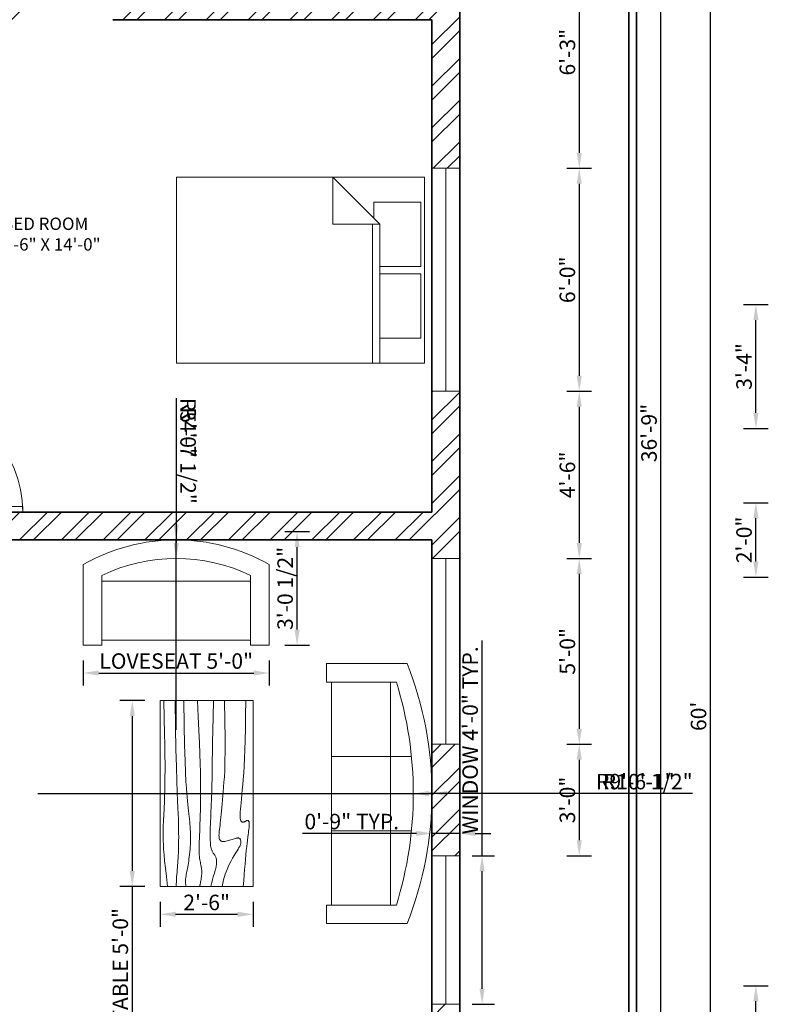
# Model space of a CAD drawing. Units: inches. Extents: x 468 to 1096, y 138 to 946.
# Tile 5 of 6: x 854 to 1096, y 448 to 766. Entities that reach past the tile are written whole.
import ezdxf

# ---------------------------------------------------------------- set-up
doc = ezdxf.new("R2010")
doc.units = ezdxf.units.IN
for name, color, linetype, lineweight in [('A-ANNO-DIMS', 2, 'Continuous', 18), ('A-AREA-IDEN', 7, 'Continuous', 18), ('A-DOOR', 3, 'Continuous', 18), ('A-FURN', 8, 'Continuous', 18), ('A-GLAZ', 4, 'Continuous', 18), ('A-WALL', 7, 'Continuous', 35), ('A-WALL-PATT', 8, 'Continuous', 13), ('C-PROP', 7, 'Continuous', 35)]:
    doc.layers.add(name, color=color, linetype=linetype, lineweight=lineweight)
doc.styles.get("Standard").update_dxf_attribs({"font": 'arial.ttf'})
doc.dimstyles.new('ISO-25', dxfattribs={"dimtxt": 5, "dimasz": 5, "dimexe": 4, "dimexo": 4, "dimtad": 1, "dimdec": 1, "dimlunit": 3, "dimtxsty": 'Standard', "dimcen": 2.5, "dimadec": 0, "dimazin": 0, "dimtfac": 1, "dimtdec": 1, "dimtmove": 0, "dimatfit": 3, "dimfxl": 4, "dimfxlon": 1, "dimarcsym": 0})

# ---------------------------------------------------------------- blocks, each defined once
blk = doc.blocks.new('*U3')
for p, q in [((0, 0), (0, -6)), ((-36, 0), (-36, -6))]:
    blk.add_line(p, q)
blk.add_lwpolyline([(0, 0), (0, 36), (-1.75, 36), (-1.75, 0)], close=True)
blk.add_arc((0, 0), 36, 90, 180)
blk = doc.blocks.new('Sofa - Roundback 7 ft.')
for p, q in [((-12.00002, -32.4421), (-12.00003, -6.5971)), ((11.99997, -32.4421), (11.99998, -6.5971)), ((-36.000027, -34), (-36.000027, -11.4696)), ((35.99998, -34), (35.99998, -11.4696)), ((-35.999844, -13.3819), (35.9998, -13.3819)), ((-36.000027, -32.4421), (35.99998, -32.4421))]:
    blk.add_line(p, q)
for points in [[(-36.000027, -34), (-42.000027, -34), (-42.000027, -8)], [(41.99998, -8), (41.99998, -34), (35.99998, -34)]]:
    blk.add_lwpolyline(points)
for centre, radius, start, end in [((0, -114.25), 114.25, 68.43141, 111.5686), ((-0.00001, -127.1968), 121.1968, 72.72033, 107.2797)]:
    blk.add_arc(centre, radius, start, end)
blk = doc.blocks.new('Sofa - Roundback Loveseat 5 ft.')
for p, q in [((0, -32.44198), (0, -5.99998)), ((-24, -33.99998), (-24, -11.46958)), ((24.00004, -33.99998), (24.00004, -11.46958)), ((-23.9998, -13.38178), (23.99986, -13.38178)), ((-24, -32.44198), (24.00004, -32.44198))]:
    blk.add_line(p, q)
for points in [[(-24, -33.99998), (-30, -33.99998), (-30, -7.99998)], [(30.00004, -7.99998), (30.00004, -33.99998), (24.00004, -33.99998)]]:
    blk.add_lwpolyline(points)
for centre, radius, start, end in [((0, -60.24998), 60.24998, 60.13715, 119.8628), ((0, -61.38438), 55.38444, 64.32083, 115.6792)]:
    blk.add_arc(centre, radius, start, end)
blk = doc.blocks.new('Table - Rectangular Woodgrain 60 x 30 in.')
for p, q in [((0, 0), (0, -30)), ((60, 0), (0, 0)), ((60, -30), (60, 0)), ((0, -30), (60, -30))]:
    blk.add_line(p, q)
for points in [[(0, -2.4), (4.8155, -2.418), (9.0302, -2.4688), (12.709, -2.5477), (15.9167, -2.65), (18.7181, -2.7711), (21.1781, -2.9063), (23.3616, -3.0508), (25.3333, -3.2), (27.1477, -3.3495), (28.8172, -3.4958), (30.3437, -3.636), (31.7291, -3.7667), (32.9756, -3.8849), (34.0849, -3.9875), (35.059, -4.0714), (35.9, -4.1334), (36.6114, -4.1711), (37.2041, -4.1854), (37.6906, -4.1779), (38.0833, -4.15), (38.3948, -4.1034), (38.6375, -4.0396), (38.8239, -3.9602), (38.9666, -3.8667), (39.0764, -3.7608), (39.1573, -3.6448), (39.2116, -3.521), (39.2416, -3.3917), (39.2498, -3.2593), (39.2385, -3.1261), (39.21, -2.9944), (39.1666, -2.8667), (39.111, -2.7447), (39.0468, -2.6281), (38.978, -2.5163), (38.9083, -2.4083), (38.8418, -2.3035), (38.7823, -2.201), (38.7337, -2.1001), (38.7, -2), (38.6844, -1.9003), (38.6875, -1.8021), (38.7094, -1.707), (38.75, -1.6167), (38.8094, -1.5326), (38.8875, -1.4563), (38.9844, -1.3893), (39.1, -1.3333), (39.2351, -1.2896), (39.3937, -1.2583), (39.5804, -1.2396), (39.8, -1.2333), (40.057, -1.2396), (40.3562, -1.2583), (40.7023, -1.2896), (41.1, -1.3333), (41.5547, -1.3895), (42.0755, -1.4573), (42.6721, -1.5361), (43.3542, -1.625), (44.1316, -1.7233), (45.014, -1.8302), (46.0114, -1.9449), (47.1333, -2.0667), (48.3862, -2.1947), (49.7625, -2.3281), (51.2513, -2.4663), (52.8416, -2.6083), (54.5226, -2.7535), (56.2833, -2.9011), (58.1127, -3.0501), (60, -3.2)], [(0, -9.2), (6.5759, -9.0858), (11.9385, -9.0365), (16.2527, -9.0418), (19.6833, -9.0917), (22.3952, -9.1759), (24.5531, -9.2844), (26.322, -9.4069), (27.8666, -9.5333), (29.3241, -9.6553), (30.7203, -9.7719), (32.0532, -9.8837), (33.3208, -9.9917), (34.5213, -10.0965), (35.6526, -10.199), (36.7128, -10.2999), (37.7, -10.4), (38.6129, -10.4996), (39.4531, -10.5969), (40.223, -10.6895), (40.925, -10.775), (41.5613, -10.8512), (42.1344, -10.9156), (42.6465, -10.966), (43.1, -11), (43.4976, -11.0158), (43.8437, -11.0136), (44.143, -10.9942), (44.4, -10.9583), (44.6195, -10.9069), (44.8062, -10.8406), (44.9648, -10.7603), (45.1, -10.6667), (45.2155, -10.5598), (45.3114, -10.4365), (45.3871, -10.2929), (45.4416, -10.125), (45.4743, -9.929), (45.4844, -9.7011), (45.4709, -9.4371), (45.4333, -9.1333), (45.3716, -8.7883), (45.2896, -8.4104), (45.1919, -8.0107), (45.0833, -7.6), (44.9685, -7.1893), (44.8521, -6.7896), (44.7388, -6.4117), (44.6333, -6.0667), (44.54, -5.7628), (44.4614, -5.4979), (44.4001, -5.2675), (44.3583, -5.0667), (44.3384, -4.8909), (44.3427, -4.7354), (44.3736, -4.5956), (44.4333, -4.4667), (44.5236, -4.3453), (44.6427, -4.2333), (44.7884, -4.1339), (44.9583, -4.05), (45.1501, -3.9849), (45.3614, -3.9417), (45.59, -3.9234), (45.8333, -3.9333), (46.0915, -3.9749), (46.3734, -4.0531), (46.6906, -4.1736), (47.0542, -4.3417), (47.4756, -4.5629), (47.9661, -4.8427), (48.5372, -5.1866), (49.2, -5.6), (49.9676, -6.0844), (50.8594, -6.625), (51.8965, -7.2031), (53.1, -7.8), (54.491, -8.3969), (56.0906, -8.975), (57.9199, -9.5156), (60, -10)], [(0, -12.8), (5.1847, -12.9322), (9.6213, -13.0323), (13.3963, -13.1059), (16.5958, -13.1583), (19.3063, -13.1952), (21.614, -13.2219), (23.6054, -13.2439), (25.3666, -13.2667), (26.9728, -13.2947), (28.4531, -13.3281), (29.8256, -13.3663), (31.1083, -13.4083), (32.3191, -13.4535), (33.476, -13.501), (34.597, -13.5501), (35.7, -13.6), (36.7984, -13.6497), (37.8875, -13.6979), (38.9578, -13.743), (40, -13.7833), (41.0047, -13.8174), (41.9625, -13.8438), (42.864, -13.8607), (43.7, -13.8667), (44.4631, -13.8604), (45.1552, -13.8417), (45.7801, -13.8104), (46.3416, -13.7667), (46.8439, -13.7104), (47.2906, -13.6417), (47.6858, -13.5604), (48.0333, -13.4667), (48.3375, -13.3608), (48.6042, -13.2448), (48.8396, -13.121), (49.05, -12.9917), (49.2417, -12.8593), (49.4208, -12.7261), (49.5937, -12.5944), (49.7667, -12.4667), (49.9452, -12.3451), (50.1323, -12.2313), (50.3303, -12.1268), (50.5416, -12.0333), (50.7686, -11.9524), (51.0135, -11.8854), (51.2788, -11.8341), (51.5666, -11.8), (51.8785, -11.7843), (52.2116, -11.7865), (52.562, -11.8059), (52.926, -11.8417), (53.2998, -11.8931), (53.6795, -11.9594), (54.0614, -12.0397), (54.4416, -12.1333), (54.8223, -12.2401), (55.2293, -12.3625), (55.6942, -12.5037), (56.2489, -12.6667), (56.9251, -12.8547), (57.7545, -13.0708), (58.7689, -13.3182), (60, -13.6)], [(0, -18), (5.124, -17.7273), (9.6609, -17.5057), (13.6705, -17.3303), (17.2125, -17.1958), (20.3467, -17.0973), (23.1328, -17.0297), (25.6307, -16.9878), (27.9, -16.9667), (29.9928, -16.9617), (31.9302, -16.9703), (33.7254, -16.9907), (35.3917, -17.0208), (36.9423, -17.0588), (38.3906, -17.1026), (39.7499, -17.1503), (41.0333, -17.2), (42.2519, -17.2496), (43.4073, -17.2969), (44.4986, -17.3395), (45.525, -17.375), (46.4858, -17.4012), (47.3802, -17.4156), (48.2074, -17.416), (48.9667, -17.4), (49.6583, -17.3662), (50.2872, -17.3167), (50.8595, -17.2547), (51.3812, -17.1833), (51.8584, -17.1057), (52.2971, -17.025), (52.7034, -16.9443), (53.0833, -16.8667), (53.443, -16.7951), (53.789, -16.7313), (54.128, -16.6768), (54.4666, -16.6334), (54.8115, -16.6024), (55.1693, -16.5854), (55.5465, -16.5841), (55.95, -16.6), (56.3828, -16.6337), (56.8346, -16.6823), (57.2915, -16.7418), (57.7396, -16.8084), (58.165, -16.878), (58.5539, -16.9469), (58.8924, -17.0111), (59.1666, -17.0667), (59.3679, -17.1107), (59.5078, -17.1438), (59.6032, -17.1675), (59.6708, -17.1833), (59.7275, -17.193), (59.7901, -17.1979), (59.8753, -17.1998), (60, -17.2)], [(0, -22.4), (8.0098, -22.2501), (14.4094, -22.1011), (19.4168, -21.9535), (23.25, -21.8083), (26.1269, -21.6663), (28.2656, -21.5281), (29.884, -21.3947), (31.2, -21.2667), (32.3967, -21.1448), (33.5172, -21.0292), (34.5697, -20.9198), (35.5625, -20.8167), (36.5037, -20.7198), (37.4015, -20.6292), (38.2642, -20.5448), (39.1, -20.4667), (39.9164, -20.3951), (40.7187, -20.3313), (41.5117, -20.2768), (42.3, -20.2333), (43.0883, -20.2024), (43.8812, -20.1854), (44.6836, -20.1841), (45.5, -20.2), (46.3328, -20.234), (47.1747, -20.2844), (48.0163, -20.3488), (48.8479, -20.425), (49.66, -20.5106), (50.4429, -20.6031), (51.1872, -20.7004), (51.8833, -20.8), (52.5246, -20.8999), (53.1166, -20.9995), (53.6681, -21.0983), (54.1875, -21.1958), (54.6834, -21.2919), (55.1646, -21.3859), (55.6394, -21.4777), (56.1167, -21.5667), (56.6028, -21.6515), (57.0961, -21.7266), (57.5929, -21.7852), (58.0896, -21.8208), (58.5823, -21.8268), (59.0674, -21.7964), (59.5412, -21.723), (60, -21.6)], [(0, -25.2), (8.6355, -25.0504), (15.7026, -24.9031), (21.4049, -24.7606), (25.9458, -24.625), (29.529, -24.4988), (32.3578, -24.3844), (34.6359, -24.284), (36.5667, -24.2), (38.3213, -24.1341), (39.9417, -24.0854), (41.437, -24.0523), (42.8167, -24.0333), (44.0901, -24.0268), (45.2667, -24.0313), (46.3557, -24.0451), (47.3667, -24.0667), (48.309, -24.0947), (49.1928, -24.1287), (50.0284, -24.168), (50.826, -24.2125), (51.5959, -24.2617), (52.3483, -24.3151), (53.0935, -24.3725), (53.8417, -24.4334), (54.6009, -24.497), (55.3699, -24.561), (56.1454, -24.6226), (56.9239, -24.6792), (57.7021, -24.7279), (58.4764, -24.7662), (59.2435, -24.7911), (60, -24.8)], [(0, -28.8), (5.6867, -28.6681), (10.45, -28.5698), (14.407, -28.5012), (17.675, -28.4584), (20.3711, -28.4374), (22.6125, -28.4344), (24.5164, -28.4455), (26.2, -28.4667), (27.762, -28.4947), (29.2276, -28.5281), (30.6033, -28.5663), (31.8958, -28.6084), (33.1118, -28.6535), (34.2578, -28.7011), (35.3405, -28.7501), (36.3666, -28.8), (37.3443, -28.8497), (38.288, -28.8974), (39.2137, -28.9412), (40.1375, -28.9792), (41.0753, -29.0093), (42.0432, -29.0297), (43.0572, -29.0384), (44.1333, -29.0333), (45.2936, -29.0114), (46.5843, -28.9641), (48.0579, -28.8816), (49.7666, -28.7542), (51.7629, -28.5721), (54.0989, -28.3255), (56.8272, -28.0048), (60, -27.6)]]:
    blk.add_lwpolyline(points)
blk = doc.blocks.new('Bed - Queen')
for p, q in [((0, -80.00003), (0, 0)), ((0, 0), (59.99999, 0)), ((59.99999, 0), (59.99999, -80.00003)), ((7.99999, -1.2), (28.79998, -1.2)), ((7.99999, -14.4), (7.99999, -1.2)), ((28.79998, -1.2), (28.79998, -14.4)), ((31.19999, -1.2), (51.99999, -1.2)), ((31.19999, -14.4), (31.19999, -1.2)), ((51.99999, -1.2), (51.99999, -16.4)), ((0, -14.4), (44.8, -14.4)), ((59.99999, -29.6), (44.8, -14.4)), ((44.8, -14.4), (44.8, -29.6)), ((44.8, -16.8), (0, -16.8)), ((51.99999, -16.4), (46.79936, -16.4)), ((44.8, -29.6), (59.99999, -29.6)), ((59.99999, -80.00003), (0, -80.00003))]:
    blk.add_line(p, q)
blk = doc.blocks.new('*D26')
at = {"layer": 'A-ANNO-DIMS', "color": 0, "lineweight": -2, "transparency": 16777216}
for p, q in [((1073, 901.16), (1081, 901.16)), ((1077, 186.16), (1077, 896.16)), ((1073, 181.16), (1081, 181.16))]:
    blk.add_line(p, q, dxfattribs=at)
at = {"layer": 'A-ANNO-DIMS', "color": 0, "transparency": 16777216}
for points in [[(1076.17, 896.16), (1077.83, 896.16), (1077, 901.16)], [(1076.17, 186.16), (1077.83, 186.16), (1077, 181.16)]]:
    blk.add_solid(points, dxfattribs=at)
at = {"layer": 'Defpoints', "color": 0, "transparency": 16777216}
for p in [(1053.13, 901.16), (1077, 901.16), (1053.13, 181.16)]:
    blk.add_point(p, dxfattribs=at)
at = {"layer": 'A-ANNO-DIMS', "color": 0, "transparency": 16777216, "insert": (1073.82, 541.16), "char_height": 5, "attachment_point": 5, "rotation": 90}
blk.add_mtext("60'", dxfattribs=at)
blk = doc.blocks.new('*D28')
at = {"layer": 'A-ANNO-DIMS', "color": 0, "lineweight": -2, "transparency": 16777216}
for p, q in [((1057.13, 853.16), (1065.02, 853.16)), ((1061.02, 417.16), (1061.02, 848.16)), ((1057.13, 412.16), (1065.02, 412.16))]:
    blk.add_line(p, q, dxfattribs=at)
at = {"layer": 'A-ANNO-DIMS', "color": 0, "transparency": 16777216}
for points in [[(1060.18, 848.16), (1061.85, 848.16), (1061.02, 853.16)], [(1060.18, 417.16), (1061.85, 417.16), (1061.02, 412.16)]]:
    blk.add_solid(points, dxfattribs=at)
at = {"layer": 'Defpoints', "color": 0, "transparency": 16777216}
for p in [(1053.13, 853.16), (1061.02, 853.16), (1053.13, 412.16)]:
    blk.add_point(p, dxfattribs=at)
at = {"layer": 'A-ANNO-DIMS', "color": 0, "transparency": 16777216, "insert": (1057.84, 632.66), "char_height": 5, "attachment_point": 5, "rotation": 90}
blk.add_mtext('36\'-9"', dxfattribs=at)
blk = doc.blocks.new('WIN-48-W9')
for p, q in [((0, 0), (0, 9)), ((48, 0), (48, 9)), ((0, 4.5), (48, 4.5))]:
    blk.add_line(p, q)
blk = doc.blocks.new('*D43')
at = {"layer": 'A-ANNO-DIMS', "color": 0, "lineweight": -2, "transparency": 16777216}
for p, q in [((1003.33, 496.16), (1003.33, 565.68)), ((1000.13, 496.16), (1007.33, 496.16)), ((1003.33, 453.16), (1003.33, 491.16)), ((1000.13, 448.16), (1007.33, 448.16))]:
    blk.add_line(p, q, dxfattribs=at)
at = {"layer": 'A-ANNO-DIMS', "color": 0, "transparency": 16777216}
for points in [[(1002.5, 491.16), (1004.16, 491.16), (1003.33, 496.16)], [(1002.5, 453.16), (1004.16, 453.16), (1003.33, 448.16)]]:
    blk.add_solid(points, dxfattribs=at)
at = {"layer": 'Defpoints', "color": 0, "transparency": 16777216}
for p in [(996.13, 496.16), (1003.33, 496.16), (996.13, 448.16)]:
    blk.add_point(p, dxfattribs=at)
at = {"layer": 'A-ANNO-DIMS', "color": 0, "transparency": 16777216, "insert": (1000.12, 533.42), "char_height": 5, "attachment_point": 5, "rotation": 90}
blk.add_mtext('WINDOW 4\'-0" TYP.', dxfattribs=at)
blk = doc.blocks.new('*D44')
at = {"layer": 'A-ANNO-DIMS', "color": 0, "lineweight": -2, "transparency": 16777216}
for p, q in [((987.13, 500.16), (987.13, 507.36)), ((996.13, 500.16), (996.13, 507.36)), ((982.13, 503.36), (945.4, 503.36)), ((996.13, 503.36), (987.13, 503.36)), ((1001.13, 503.36), (1006.13, 503.36))]:
    blk.add_line(p, q, dxfattribs=at)
at = {"layer": 'A-ANNO-DIMS', "color": 0, "transparency": 16777216}
for points in [[(982.13, 504.19), (982.13, 502.53), (987.13, 503.36)], [(1001.13, 504.19), (1001.13, 502.53), (996.13, 503.36)]]:
    blk.add_solid(points, dxfattribs=at)
at = {"layer": 'Defpoints', "color": 0, "transparency": 16777216}
for p in [(987.13, 503.36), (987.13, 496.16), (996.13, 496.16)]:
    blk.add_point(p, dxfattribs=at)
at = {"layer": 'A-ANNO-DIMS', "color": 0, "transparency": 16777216, "insert": (961.27, 506.54), "char_height": 5, "attachment_point": 5}
blk.add_mtext('0\'-9" TYP.', dxfattribs=at)
blk = doc.blocks.new('*D49')
at = {"layer": 'A-ANNO-DIMS', "color": 0, "lineweight": -2, "transparency": 16777216}
for p, q in [((874.63, 559.16), (874.63, 551.16)), ((934.63, 559.16), (934.63, 551.16)), ((879.63, 555.16), (929.63, 555.16))]:
    blk.add_line(p, q, dxfattribs=at)
at = {"layer": 'A-ANNO-DIMS', "color": 0, "transparency": 16777216}
for points in [[(879.63, 555.99), (879.63, 554.33), (874.63, 555.16)], [(929.63, 555.99), (929.63, 554.33), (934.63, 555.16)]]:
    blk.add_solid(points, dxfattribs=at)
at = {"layer": 'Defpoints', "color": 0, "transparency": 16777216}
for p in [(874.63, 564.16), (934.63, 564.16), (934.63, 555.16)]:
    blk.add_point(p, dxfattribs=at)
at = {"layer": 'A-ANNO-DIMS', "color": 0, "transparency": 16777216, "insert": (904.63, 558.37), "char_height": 5, "attachment_point": 5}
blk.add_mtext('LOVESEAT 5\'-0"', dxfattribs=at)
blk = doc.blocks.new('*D50')
at = {"layer": 'A-ANNO-DIMS', "color": 0, "lineweight": -2, "transparency": 16777216}
for p, q in [((939.63, 600.83), (947.63, 600.83)), ((943.63, 569.16), (943.63, 595.83)), ((939.63, 564.16), (947.63, 564.16))]:
    blk.add_line(p, q, dxfattribs=at)
at = {"layer": 'A-ANNO-DIMS', "color": 0, "transparency": 16777216}
for points in [[(942.8, 595.83), (944.46, 595.83), (943.63, 600.83)], [(942.8, 569.16), (944.46, 569.16), (943.63, 564.16)]]:
    blk.add_solid(points, dxfattribs=at)
at = {"layer": 'Defpoints', "color": 0, "transparency": 16777216}
for p in [(934.63, 600.83), (943.63, 600.83), (934.63, 564.16)]:
    blk.add_point(p, dxfattribs=at)
at = {"layer": 'A-ANNO-DIMS', "color": 0, "transparency": 16777216, "insert": (940.42, 582.49), "char_height": 5, "attachment_point": 5, "rotation": 90}
blk.add_mtext('3\'-0 1/2"', dxfattribs=at)
blk = doc.blocks.new('*D51')
at = {"layer": 'A-ANNO-DIMS', "color": 0, "lineweight": -2, "transparency": 16777216}
for p, q in [((894.45, 546.23), (886.45, 546.23)), ((890.45, 541.23), (890.45, 491.23)), ((894.45, 486.23), (886.45, 486.23)), ((890.45, 486.23), (890.45, 411.4))]:
    blk.add_line(p, q, dxfattribs=at)
at = {"layer": 'A-ANNO-DIMS', "color": 0, "transparency": 16777216}
for points in [[(889.62, 541.23), (891.28, 541.23), (890.45, 546.23)], [(889.62, 491.23), (891.28, 491.23), (890.45, 486.23)]]:
    blk.add_solid(points, dxfattribs=at)
at = {"layer": 'Defpoints', "color": 0, "transparency": 16777216}
for p in [(899.45, 546.23), (890.45, 486.23), (899.45, 486.23)]:
    blk.add_point(p, dxfattribs=at)
at = {"layer": 'A-ANNO-DIMS', "color": 0, "transparency": 16777216, "insert": (887.24, 446.31), "char_height": 5, "attachment_point": 5, "rotation": 90}
blk.add_mtext('LOUNGE TABLE 5\'-0"', dxfattribs=at)
blk = doc.blocks.new('*D52')
at = {"layer": 'A-ANNO-DIMS', "color": 0, "lineweight": -2, "transparency": 16777216}
for p, q in [((899.45, 481.23), (899.45, 473.23)), ((929.45, 481.23), (929.45, 473.23)), ((904.45, 477.23), (924.45, 477.23))]:
    blk.add_line(p, q, dxfattribs=at)
at = {"layer": 'A-ANNO-DIMS', "color": 0, "transparency": 16777216}
for points in [[(904.45, 478.06), (904.45, 476.39), (899.45, 477.23)], [(924.45, 478.06), (924.45, 476.39), (929.45, 477.23)]]:
    blk.add_solid(points, dxfattribs=at)
at = {"layer": 'Defpoints', "color": 0, "transparency": 16777216}
for p in [(899.45, 486.23), (929.45, 486.23), (929.45, 477.23)]:
    blk.add_point(p, dxfattribs=at)
at = {"layer": 'A-ANNO-DIMS', "color": 0, "transparency": 16777216, "insert": (914.45, 480.41), "char_height": 5, "attachment_point": 5}
blk.add_mtext('2\'-6"', dxfattribs=at)
blk = doc.blocks.new('*D64')
at = {"layer": 'A-ANNO-DIMS', "color": 0, "lineweight": -2, "transparency": 16777216}
for p, q in [((854.13, 146.61), (854.13, 138.61)), ((884.13, 146.61), (884.13, 138.61)), ((859.13, 142.61), (879.13, 142.61))]:
    blk.add_line(p, q, dxfattribs=at)
at = {"layer": 'A-ANNO-DIMS', "color": 0, "transparency": 16777216}
for points in [[(859.13, 143.44), (859.13, 141.78), (854.13, 142.61)], [(879.13, 143.44), (879.13, 141.78), (884.13, 142.61)]]:
    blk.add_solid(points, dxfattribs=at)
at = {"layer": 'Defpoints', "color": 0, "transparency": 16777216}
for p in [(854.13, 766.16), (884.13, 766.16), (884.13, 142.61)]:
    blk.add_point(p, dxfattribs=at)
at = {"layer": 'A-ANNO-DIMS', "color": 0, "transparency": 16777216, "insert": (869.13, 145.79), "char_height": 5, "attachment_point": 5}
blk.add_mtext('2\'-6"', dxfattribs=at)
blk = doc.blocks.new('*D67')
at = {"layer": 'A-ANNO-DIMS', "color": 0, "lineweight": -2, "transparency": 16777216}
for p, q in [((1030.68, 718.16), (1038.68, 718.16)), ((1034.68, 713.16), (1034.68, 651.16)), ((1030.68, 646.16), (1038.68, 646.16))]:
    blk.add_line(p, q, dxfattribs=at)
at = {"layer": 'A-ANNO-DIMS', "color": 0, "transparency": 16777216}
for points in [[(1033.85, 713.16), (1035.51, 713.16), (1034.68, 718.16)], [(1033.85, 651.16), (1035.51, 651.16), (1034.68, 646.16)]]:
    blk.add_solid(points, dxfattribs=at)
at = {"layer": 'Defpoints', "color": 0, "transparency": 16777216}
for p in [(996.13, 718.16), (996.13, 646.16), (1034.68, 646.16)]:
    blk.add_point(p, dxfattribs=at)
at = {"layer": 'A-ANNO-DIMS', "color": 0, "transparency": 16777216, "insert": (1031.5, 682.16), "char_height": 5, "attachment_point": 5, "rotation": 90}
blk.add_mtext('6\'-0"', dxfattribs=at)
blk = doc.blocks.new('*D68')
at = {"layer": 'A-ANNO-DIMS', "color": 0, "lineweight": -2, "transparency": 16777216}
for p, q in [((1030.68, 592.16), (1038.68, 592.16)), ((1034.68, 587.16), (1034.68, 537.16)), ((1030.68, 532.16), (1038.68, 532.16))]:
    blk.add_line(p, q, dxfattribs=at)
at = {"layer": 'A-ANNO-DIMS', "color": 0, "transparency": 16777216}
for points in [[(1033.85, 587.16), (1035.51, 587.16), (1034.68, 592.16)], [(1033.85, 537.16), (1035.51, 537.16), (1034.68, 532.16)]]:
    blk.add_solid(points, dxfattribs=at)
at = {"layer": 'Defpoints', "color": 0, "transparency": 16777216}
for p in [(996.13, 592.16), (996.13, 532.16), (1034.68, 532.16)]:
    blk.add_point(p, dxfattribs=at)
at = {"layer": 'A-ANNO-DIMS', "color": 0, "transparency": 16777216, "insert": (1031.5, 562.16), "char_height": 5, "attachment_point": 5, "rotation": 90}
blk.add_mtext('5\'-0"', dxfattribs=at)
blk = doc.blocks.new('*D69')
at = {"layer": 'A-ANNO-DIMS', "color": 0, "lineweight": -2, "transparency": 16777216}
for p, q in [((1030.68, 532.16), (1038.68, 532.16)), ((1034.68, 527.16), (1034.68, 501.16)), ((1030.68, 496.16), (1038.68, 496.16))]:
    blk.add_line(p, q, dxfattribs=at)
at = {"layer": 'A-ANNO-DIMS', "color": 0, "transparency": 16777216}
for points in [[(1033.85, 527.16), (1035.51, 527.16), (1034.68, 532.16)], [(1033.85, 501.16), (1035.51, 501.16), (1034.68, 496.16)]]:
    blk.add_solid(points, dxfattribs=at)
at = {"layer": 'Defpoints', "color": 0, "transparency": 16777216}
for p in [(996.13, 532.16), (996.13, 496.16), (1034.68, 496.16)]:
    blk.add_point(p, dxfattribs=at)
at = {"layer": 'A-ANNO-DIMS', "color": 0, "transparency": 16777216, "insert": (1031.5, 514.16), "char_height": 5, "attachment_point": 5, "rotation": 90}
blk.add_mtext('3\'-0"', dxfattribs=at)
blk = doc.blocks.new('*D72')
at = {"layer": 'A-ANNO-DIMS', "color": 0, "lineweight": -2, "transparency": 16777216}
for p, q in [((1030.68, 793.16), (1038.68, 793.16)), ((1034.68, 788.16), (1034.68, 723.16)), ((1030.68, 718.16), (1038.68, 718.16))]:
    blk.add_line(p, q, dxfattribs=at)
at = {"layer": 'A-ANNO-DIMS', "color": 0, "transparency": 16777216}
for points in [[(1033.85, 788.16), (1035.51, 788.16), (1034.68, 793.16)], [(1033.85, 723.16), (1035.51, 723.16), (1034.68, 718.16)]]:
    blk.add_solid(points, dxfattribs=at)
at = {"layer": 'Defpoints', "color": 0, "transparency": 16777216}
for p in [(996.13, 793.16), (996.13, 718.16), (1034.68, 718.16)]:
    blk.add_point(p, dxfattribs=at)
at = {"layer": 'A-ANNO-DIMS', "color": 0, "transparency": 16777216, "insert": (1031.5, 755.66), "char_height": 5, "attachment_point": 5, "rotation": 90}
blk.add_mtext('6\'-3"', dxfattribs=at)
blk = doc.blocks.new('*D73')
at = {"layer": 'A-ANNO-DIMS', "color": 0, "lineweight": -2, "transparency": 16777216}
for p, q in [((1030.68, 646.16), (1038.68, 646.16)), ((1034.68, 641.16), (1034.68, 597.16)), ((1030.68, 592.16), (1038.68, 592.16))]:
    blk.add_line(p, q, dxfattribs=at)
at = {"layer": 'A-ANNO-DIMS', "color": 0, "transparency": 16777216}
for points in [[(1033.85, 641.16), (1035.51, 641.16), (1034.68, 646.16)], [(1033.85, 597.16), (1035.51, 597.16), (1034.68, 592.16)]]:
    blk.add_solid(points, dxfattribs=at)
at = {"layer": 'Defpoints', "color": 0, "transparency": 16777216}
for p in [(996.13, 646.16), (996.13, 592.16), (1034.68, 592.16)]:
    blk.add_point(p, dxfattribs=at)
at = {"layer": 'A-ANNO-DIMS', "color": 0, "transparency": 16777216, "insert": (1031.5, 619.16), "char_height": 5, "attachment_point": 5, "rotation": 90}
blk.add_mtext('4\'-6"', dxfattribs=at)
blk = doc.blocks.new('*D76')
at = {"layer": 'A-ANNO-DIMS', "color": 0, "lineweight": -2, "transparency": 16777216}
for p, q in [((1087.68, 454.16), (1095.68, 454.16)), ((1091.68, 423.16), (1091.68, 449.16)), ((1087.68, 418.16), (1095.68, 418.16))]:
    blk.add_line(p, q, dxfattribs=at)
at = {"layer": 'A-ANNO-DIMS', "color": 0, "transparency": 16777216}
for points in [[(1090.85, 449.16), (1092.51, 449.16), (1091.68, 454.16)], [(1090.85, 423.16), (1092.51, 423.16), (1091.68, 418.16)]]:
    blk.add_solid(points, dxfattribs=at)
at = {"layer": 'Defpoints', "color": 0, "transparency": 16777216}
for p in [(687.13, 454.16), (1091.68, 454.16), (687.13, 418.16)]:
    blk.add_point(p, dxfattribs=at)
at = {"layer": 'A-ANNO-DIMS', "color": 0, "transparency": 16777216, "insert": (1088.5, 436.16), "char_height": 5, "attachment_point": 5, "rotation": 90}
blk.add_mtext('3\'-0"', dxfattribs=at)
blk = doc.blocks.new('*D82')
at = {"layer": 'A-ANNO-DIMS', "color": 0, "lineweight": -2, "transparency": 16777216}
for p, q in [((1087.68, 674.16), (1095.68, 674.16)), ((1091.68, 639.16), (1091.68, 669.16)), ((1087.68, 634.16), (1095.68, 634.16))]:
    blk.add_line(p, q, dxfattribs=at)
at = {"layer": 'A-ANNO-DIMS', "color": 0, "transparency": 16777216}
for points in [[(1090.85, 669.16), (1092.51, 669.16), (1091.68, 674.16)], [(1090.85, 639.16), (1092.51, 639.16), (1091.68, 634.16)]]:
    blk.add_solid(points, dxfattribs=at)
at = {"layer": 'Defpoints', "color": 0, "transparency": 16777216}
for p in [(687.13, 674.16), (1091.68, 674.16), (687.13, 634.16)]:
    blk.add_point(p, dxfattribs=at)
at = {"layer": 'A-ANNO-DIMS', "color": 0, "transparency": 16777216, "insert": (1088.5, 654.16), "char_height": 5, "attachment_point": 5, "rotation": 90}
blk.add_mtext('3\'-4"', dxfattribs=at)
blk = doc.blocks.new('*D86')
at = {"layer": 'A-ANNO-DIMS', "color": 0, "lineweight": -2, "transparency": 16777216}
for p, q in [((1087.68, 610.16), (1095.68, 610.16)), ((1091.68, 591.16), (1091.68, 605.16)), ((1087.68, 586.16), (1095.68, 586.16))]:
    blk.add_line(p, q, dxfattribs=at)
at = {"layer": 'A-ANNO-DIMS', "color": 0, "transparency": 16777216}
for points in [[(1090.85, 605.16), (1092.51, 605.16), (1091.68, 610.16)], [(1090.85, 591.16), (1092.51, 591.16), (1091.68, 586.16)]]:
    blk.add_solid(points, dxfattribs=at)
at = {"layer": 'Defpoints', "color": 0, "transparency": 16777216}
for p in [(579.13, 610.16), (1091.68, 610.16), (579.13, 586.16)]:
    blk.add_point(p, dxfattribs=at)
at = {"layer": 'A-ANNO-DIMS', "color": 0, "transparency": 16777216, "insert": (1088.5, 598.16), "char_height": 5, "attachment_point": 5, "rotation": 90}
blk.add_mtext('2\'-0"', dxfattribs=at)
blk = doc.blocks.new('*D87')
at = {"layer": 'A-ANNO-DIMS', "color": 0, "lineweight": -2, "transparency": 16777216}
for p, q in [((859.93, 516.23), (981.13, 516.23)), ((1065.45, 516.24), (986.13, 516.23))]:
    blk.add_line(p, q, dxfattribs=at)
at = {"layer": 'A-ANNO-DIMS', "color": 0, "transparency": 16777216}
blk.add_solid([(986.13, 517.07), (986.13, 515.4), (981.13, 516.23)], dxfattribs=at)
at = {"layer": 'Defpoints', "color": 0, "transparency": 16777216}
for p in [(859.93, 516.23), (981.13, 516.23)]:
    blk.add_point(p, dxfattribs=at)
at = {"layer": 'A-ANNO-DIMS', "color": 0, "transparency": 16777216, "insert": (1053.85, 519.41), "char_height": 5, "attachment_point": 5, "rotation": 0.0002}
blk.add_mtext('R10\'-1"', dxfattribs=at)
blk = doc.blocks.new('*D88')
at = {"layer": 'A-ANNO-DIMS', "color": 0, "lineweight": -2, "transparency": 16777216}
for p, q in [((872.88, 516.23), (987.13, 516.23)), ((1071.17, 516.23), (992.13, 516.23))]:
    blk.add_line(p, q, dxfattribs=at)
at = {"layer": 'A-ANNO-DIMS', "color": 0, "transparency": 16777216}
blk.add_solid([(992.13, 517.07), (992.13, 515.4), (987.13, 516.23)], dxfattribs=at)
at = {"layer": 'Defpoints', "color": 0, "transparency": 16777216}
for p in [(872.88, 516.23), (987.13, 516.23)]:
    blk.add_point(p, dxfattribs=at)
at = {"layer": 'A-ANNO-DIMS', "color": 0, "transparency": 16777216, "insert": (1055.68, 519.44), "char_height": 5, "attachment_point": 5, "rotation": 359.9998}
blk.add_mtext('R9\'-6 1/2"', dxfattribs=at)
blk = doc.blocks.new('*D89')
at = {"layer": 'A-ANNO-DIMS', "color": 0, "lineweight": -2, "transparency": 16777216}
for p, q in [((904.63, 643.97), (904.63, 603.16)), ((904.63, 537.91), (904.63, 598.16))]:
    blk.add_line(p, q, dxfattribs=at)
at = {"layer": 'A-ANNO-DIMS', "color": 0, "transparency": 16777216}
blk.add_solid([(905.46, 603.16), (903.8, 603.16), (904.63, 598.16)], dxfattribs=at)
at = {"layer": 'Defpoints', "color": 0, "transparency": 16777216}
for p in [(904.63, 598.16), (904.63, 537.91)]:
    blk.add_point(p, dxfattribs=at)
at = {"layer": 'A-ANNO-DIMS', "color": 0, "transparency": 16777216, "insert": (907.81, 634.31), "char_height": 5, "attachment_point": 5, "rotation": 270.0002}
blk.add_mtext('R5\'-0"', dxfattribs=at)
blk = doc.blocks.new('*D90')
at = {"layer": 'A-ANNO-DIMS', "color": 0, "lineweight": -2, "transparency": 16777216}
for p, q in [((904.63, 640.88), (904.63, 597.16)), ((904.63, 536.78), (904.63, 592.16))]:
    blk.add_line(p, q, dxfattribs=at)
at = {"layer": 'A-ANNO-DIMS', "color": 0, "transparency": 16777216}
blk.add_solid([(905.46, 597.16), (903.8, 597.16), (904.63, 592.16)], dxfattribs=at)
at = {"layer": 'Defpoints', "color": 0, "transparency": 16777216}
for p in [(904.63, 592.16), (904.63, 536.78)]:
    blk.add_point(p, dxfattribs=at)
at = {"layer": 'A-ANNO-DIMS', "color": 0, "transparency": 16777216, "insert": (907.84, 625.39), "char_height": 5, "attachment_point": 5, "rotation": 270.0002}
blk.add_mtext('R4\'-7 1/2"', dxfattribs=at)

msp = doc.modelspace()

# ---------------------------------------------------------------- hatches: boundary and pattern name
at = {"layer": 'A-WALL-PATT'}
h = msp.add_hatch(dxfattribs=at)
h.set_pattern_fill('ANSI32', color=256)
h.paths.add_polyline_path([(696.13, 634.16), (687.13, 634.16), (650.13, 634.16), (567.13, 634.16), (567.13, 625.16), (573.13, 625.16), (573.13, 610.16), (579.13, 610.16), (579.13, 625.16), (687.13, 625.16), (687.13, 454.16), (696.13, 454.16), (696.13, 598.16), (813.13, 598.16), (813.13, 607.16), (696.13, 607.16)])
h.paths.add_polyline_path([(777.13, 688.16), (777.13, 691.16), (696.13, 691.16), (696.13, 820.16), (721.13, 820.16), (721.13, 829.16), (687.13, 829.16), (687.13, 820.16), (687.13, 674.16), (696.13, 674.16), (696.13, 682.16), (777.13, 682.16)])
h.paths.add_polyline_path([(854.13, 775.16), (822.13, 775.16), (822.13, 835.16), (884.13, 835.16), (884.13, 803.19), (888.13, 803.19), (888.13, 835.16), (987.13, 835.16), (987.13, 817.16), (996.13, 817.16), (996.13, 844.16), (987.13, 844.16), (813.13, 844.16), (813.13, 829.16), (813.13, 823.16), (813.13, 791.16), (813.13, 691.16), (813.13, 688.16), (813.13, 682.16), (813.13, 643.16), (819.13, 643.16), (822.13, 643.16), (822.13, 691.16), (822.13, 766.16), (854.13, 766.16)])
h.paths.add_polyline_path([(996.13, 775.16), (996.13, 784.16), (996.13, 793.16), (987.13, 793.16), (987.13, 775.16), (884.13, 775.16), (884.13, 766.16), (987.13, 766.16), (987.13, 718.16), (996.13, 718.16)], flags=17)
h.paths.add_polyline_path([(781.13, 829.16), (757.13, 829.16), (757.13, 820.16), (781.13, 820.16)])
h = msp.add_hatch(dxfattribs=at)
h.set_pattern_fill('ANSI32', color=256)
h.paths.add_polyline_path([(1053.13, 412.16), (1044.13, 412.16), (1044.13, 241.16), (1053.13, 241.16)])
h.paths.add_polyline_path([(996.13, 448.16), (987.13, 448.16), (987.13, 412.16), (942.13, 412.16), (942.13, 403.16), (996.13, 403.16)])
h.paths.add_polyline_path([(996.13, 532.16), (987.13, 532.16), (987.13, 496.16), (996.13, 496.16)])
h.paths.add_polyline_path([(996.13, 646.16), (987.13, 646.16), (987.13, 607.16), (813.13, 607.16), (813.13, 598.16), (822.13, 598.16), (987.13, 598.16), (987.13, 592.16), (996.13, 592.16), (996.13, 598.16), (996.13, 607.16)])
h.paths.add_polyline_path([(894.13, 412.16), (849.13, 412.16), (849.13, 403.16), (894.13, 403.16)])
h.paths.add_polyline_path([(801.13, 412.16), (744.13, 412.16), (744.13, 250.16), (744.13, 241.16), (777.13, 241.16), (777.13, 250.16), (753.13, 250.16), (753.13, 403.16), (801.13, 403.16)])
h.paths.add_polyline_path([(744.13, 412.16), (736.13, 412.16), (736.13, 403.16), (744.13, 403.16)])

# ---------------------------------------------------------------- linework, layer by layer
at = {"layer": 'A-GLAZ'}
for p, q in [((987.13, 718.16), (996.13, 718.16)), ((991.63, 646.16), (991.63, 718.16)), ((987.13, 646.16), (996.13, 646.16)), ((987.13, 592.16), (996.13, 592.16)), ((991.63, 532.16), (991.63, 592.16)), ((987.13, 532.16), (996.13, 532.16))]:
    msp.add_line(p, q, dxfattribs=at)
at = {"layer": 'A-WALL'}
for p, q in [((884.13, 766.16), (987.13, 766.16)), ((987.13, 766.16), (987.13, 607.16)), ((987.13, 607.16), (813.13, 607.16)), ((987.13, 412.16), (987.13, 598.16)), ((996.13, 403.16), (996.13, 598.16))]:
    msp.add_line(p, q, dxfattribs=at)
for points in [[(813.13, 829.16), (813.13, 844.16), (987.13, 844.16), (996.13, 844.16), (996.13, 784.16), (996.13, 775.16), (996.13, 607.16), (996.13, 598.16)], [(987.13, 598.16), (822.13, 598.16), (813.13, 598.16)]]:
    msp.add_lwpolyline(points, dxfattribs=at)
at = {"layer": 'C-PROP'}
for p, q in [((1053.13, 181.16), (1053.13, 901.16)), ((1050.72, 412.16), (1050.72, 892.16))]:
    msp.add_line(p, q, dxfattribs=at)

# ---------------------------------------------------------------- block references
at = {"layer": 'A-DOOR', "rotation": 270}
msp.add_blockref('*U3', (819.13, 607.16), dxfattribs=at)
at = {"layer": 'A-FURN', "xscale": -1, "rotation": 270}
msp.add_blockref('Bed - Queen', (984.77, 655.27), dxfattribs=at)
at = {"layer": 'A-FURN'}
msp.add_blockref('Sofa - Roundback Loveseat 5 ft.', (904.63, 598.16), dxfattribs=at)
at = {"layer": 'A-FURN', "rotation": 270}
for name, p in [('Sofa - Roundback 7 ft.', (987.13, 516.23)), ('Table - Rectangular Woodgrain 60 x 30 in.', (929.45, 546.23))]:
    msp.add_blockref(name, p, dxfattribs=at)
at = {"layer": 'A-GLAZ', "rotation": 90.0000000000004}
msp.add_blockref('WIN-48-W9', (996.13, 448.16), dxfattribs=at)

# ---------------------------------------------------------------- texts
at = {"layer": 'A-AREA-IDEN', "insert": (844.23, 702.25), "char_height": 4, "attachment_point": 1}
msp.add_mtext_dynamic_manual_height_columns('\\pxqc;BED ROOM\\P14\'-6" X 14\'-0"', width=36.2598, gutter_width=12.5, heights=[0], dxfattribs=at)

# ---------------------------------------------------------------- dimensions: what is measured, and where the dimension line sits
at = {"layer": 'A-ANNO-DIMS'}
for base, p1, p2, angle, override, picture, middle in [((1077, 901.16), (1053.13, 181.16), (1053.13, 901.16), 90, {"dimclrd": 0, "dimclre": 0, "dimclrt": 0}, '*D26', (1073.82, 541.16)), ((1061.02, 853.16), (1053.13, 412.16), (1053.13, 853.16), 90, {"dimclrd": 0, "dimclre": 0, "dimclrt": 0}, '*D28', (1057.84, 632.66)), ((1034.68, 718.16), (996.13, 793.16), (996.13, 718.16), 270, {"dimdec": 1, "dimlfac": 1, "dimrnd": 0, "dimzin": 1, "dimdsep": 46, "dimlunit": 4, "dimfrac": 2}, '*D72', (1031.5, 755.66)), ((1034.68, 646.16), (996.13, 718.16), (996.13, 646.16), 270, {"dimdec": 1, "dimlfac": 1, "dimrnd": 0, "dimzin": 1, "dimdsep": 46, "dimlunit": 4, "dimfrac": 2}, '*D67', (1031.5, 682.16)), ((1091.68, 674.16), (687.13, 634.16), (687.13, 674.16), 90, {"dimdec": 1, "dimlfac": 1, "dimrnd": 0, "dimzin": 1, "dimdsep": 46, "dimlunit": 4, "dimfrac": 2}, '*D82', (1088.5, 654.16)), ((1034.68, 592.16), (996.13, 646.16), (996.13, 592.16), 270, {"dimdec": 1, "dimlfac": 1, "dimrnd": 0, "dimzin": 1, "dimdsep": 46, "dimlunit": 4, "dimfrac": 2}, '*D73', (1031.5, 619.16)), ((1091.68, 610.16), (579.13, 586.16), (579.13, 610.16), 90, {"dimdec": 1, "dimlfac": 1, "dimrnd": 0, "dimzin": 1, "dimdsep": 46, "dimlunit": 4, "dimfrac": 2}, '*D86', (1088.5, 598.16)), ((943.63, 600.83), (934.63, 564.16), (934.63, 600.83), 90, {"dimdec": 1, "dimlfac": 1, "dimrnd": 0, "dimzin": 1, "dimdsep": 46, "dimlunit": 4, "dimfrac": 2}, '*D50', (940.42, 582.49)), ((1034.68, 532.16), (996.13, 592.16), (996.13, 532.16), 270, {"dimdec": 1, "dimlfac": 1, "dimrnd": 0, "dimzin": 1, "dimdsep": 46, "dimlunit": 4, "dimfrac": 2}, '*D68', (1031.5, 562.16)), ((1034.68, 496.16), (996.13, 532.16), (996.13, 496.16), 270, {"dimdec": 1, "dimlfac": 1, "dimrnd": 0, "dimzin": 1, "dimdsep": 46, "dimlunit": 4, "dimfrac": 2}, '*D69', (1031.5, 514.16)), ((1091.68, 454.16), (687.13, 418.16), (687.13, 454.16), 90, {"dimdec": 1, "dimlfac": 1, "dimrnd": 0, "dimzin": 1, "dimdsep": 46, "dimlunit": 4, "dimfrac": 2}, '*D76', (1088.5, 436.16))]:
    dim = msp.add_linear_dim(base=base, p1=p1, p2=p2, angle=angle, dimstyle='ISO-25', override=override, dxfattribs=at)
    dim.commit()
    dim.dimension.update_dxf_attribs({"geometry": picture, "text_midpoint": middle})
for base, p1, p2, picture, middle in [((884.13, 142.61), (854.13, 766.16), (884.13, 766.16), '*D64', (869.13, 145.79)), ((929.45, 477.23), (899.45, 486.23), (929.45, 486.23), '*D52', (914.45, 480.41))]:
    dim = msp.add_linear_dim(base=base, p1=p1, p2=p2, dimstyle='ISO-25', override={"dimdec": 1, "dimlfac": 1, "dimrnd": 0, "dimzin": 1, "dimdsep": 46, "dimlunit": 4, "dimfrac": 2}, dxfattribs=at)
    dim.commit()
    dim.dimension.update_dxf_attribs({"geometry": picture, "text_midpoint": middle})
for center, mpoint, picture, middle in [((904.6292, 537.91141), (904.629, 598.16139), '*D89', (904.62888, 634.31138)), ((904.63, 536.78), (904.63, 592.16), '*D90', (904.63, 625.39)), ((872.879196, 516.234485), (987.129196, 516.234), '*D88', (1055.679196, 516.233709)), ((859.93, 516.23), (981.13, 516.23), '*D87', (1053.85, 516.24))]:
    dim = msp.add_radius_dim(center=center, mpoint=mpoint, dimstyle='ISO-25', override={"dimdec": 1, "dimlfac": 1, "dimrnd": 0, "dimzin": 1, "dimdsep": 46, "dimlunit": 4, "dimfrac": 2}, dxfattribs=at)
    dim.commit()
    dim.dimension.update_dxf_attribs({"geometry": picture, "text_midpoint": middle, "dimtype": 164})
dim = msp.add_linear_dim(base=(934.63, 555.16), p1=(874.63, 564.16), p2=(934.63, 564.16), text='LOVESEAT <>', dimstyle='ISO-25', override={"dimdec": 1, "dimlfac": 1, "dimrnd": 0, "dimzin": 1, "dimdsep": 46, "dimlunit": 4, "dimfrac": 2}, dxfattribs=at)
dim.commit()
dim.dimension.update_dxf_attribs({"geometry": '*D49', "text_midpoint": (904.63, 558.37)})
for base, p1, p2, angle, text, picture, middle in [((1003.33, 496.16), (996.13, 448.16), (996.13, 496.16), 90, 'WINDOW <> TYP.', '*D43', (1000.12, 533.42)), ((890.45, 486.23), (899.45, 546.23), (899.45, 486.23), 270, 'LOUNGE TABLE <>', '*D51', (887.24, 446.31)), ((987.13, 503.36), (996.13, 496.16), (987.13, 496.16), 180, '<> TYP.', '*D44', (961.27, 506.54))]:
    dim = msp.add_linear_dim(base=base, p1=p1, p2=p2, angle=angle, text=text, dimstyle='ISO-25', override={"dimdec": 1, "dimlfac": 1, "dimrnd": 0, "dimzin": 1, "dimdsep": 46, "dimlunit": 4, "dimfrac": 2}, dxfattribs=at)
    dim.commit()
    dim.dimension.update_dxf_attribs({"geometry": picture, "text_midpoint": middle})

doc.saveas('drawing.dxf')
